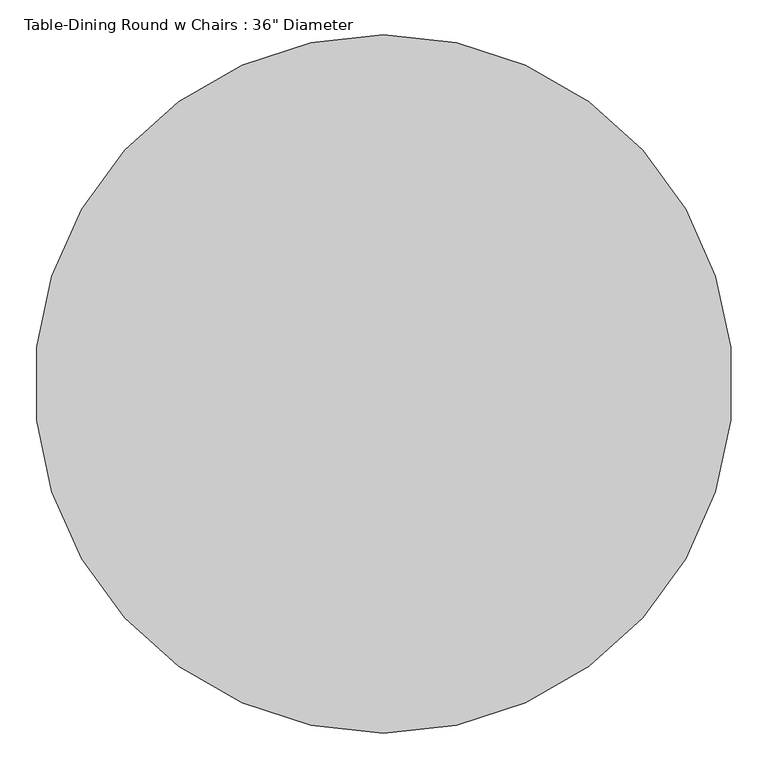
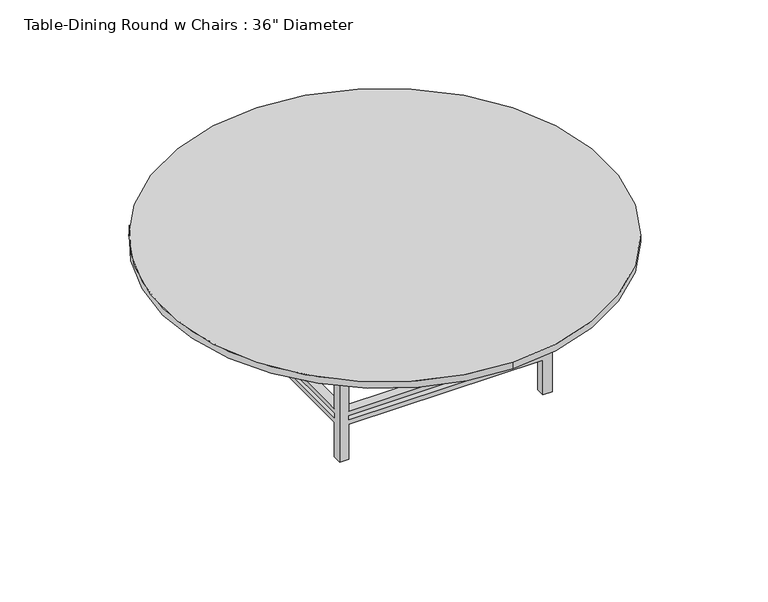
"""IFC4 building model written with IfcOpenShell, lengths in millimetres: furniture geometry."""

from ifc_helpers import new_model, si_unit, point, frame, frame_2d, origin, place, context, project, spatial, polyline, circle_curve, trimmed, segment, composite_curve, outline, extrude, faceted_brep, source, transform, mapped, element, save


def furniture_5d3b8c6f(model_context):
    return source(origin(), model_context, "Body", "SolidModel", [
        faceted_brep([(637.0819672, 348.5213115, 279.4), (637.0819672, -718.2786885, 279.4), (687.8819672, -718.2786885, 279.4), (687.8819672, 348.5213115, 279.4), (-429.7180328, -718.2786885, 279.4), (-429.7180328, -769.0786885, 279.4), (637.0819672, -769.0786885, 279.4), (-429.7180328, 348.5213115, 279.4), (-480.5180328, 348.5213115, 279.4), (-480.5180328, -718.2786885, 279.4), (637.0819672, 399.3213115, 279.4), (-429.7180328, 399.3213115, 279.4), (637.0819672, 348.5213115, 254.0), (-429.7180328, 348.5213115, 254.0), (-429.7180328, 399.3213115, 254.0), (637.0819672, 399.3213115, 254.0), (-429.7180328, -718.2786885, 254.0), (-480.5180328, -718.2786885, 254.0), (-480.5180328, 348.5213115, 254.0), (637.0819672, -718.2786885, 254.0), (637.0819672, -769.0786885, 254.0), (-429.7180328, -769.0786885, 254.0), (687.8819672, 348.5213115, 254.0), (687.8819672, -718.2786885, 254.0), (-480.5180328, 399.3213115, 647.7), (-429.7180328, 399.3213115, 647.7), (637.0819672, 399.3213115, 647.7), (687.8819672, 399.3213115, 647.7), (687.8819672, 399.3213115, 0.0), (637.0819672, 399.3213115, 0.0), (637.0819672, 399.3213115, 203.2), (-429.7180328, 399.3213115, 203.2), (-429.7180328, 399.3213115, 0.0), (-480.5180328, 399.3213115, 0.0), (-429.7180328, 399.3213115, 228.6), (637.0819672, 399.3213115, 228.6), (-480.5180328, 348.5213115, 647.7), (-480.5180328, 348.5213115, 0.0), (-480.5180328, 348.5213115, 203.2), (-480.5180328, -718.2786885, 203.2), (-480.5180328, -718.2786885, 0.0), (-480.5180328, -769.0786885, 0.0), (-480.5180328, -769.0786885, 647.7), (-480.5180328, -718.2786885, 647.7), (-480.5180328, -718.2786885, 228.6), (-480.5180328, 348.5213115, 228.6), (687.8819672, -769.0786885, 647.7), (637.0819672, -769.0786885, 647.7), (-429.7180328, -769.0786885, 647.7), (-429.7180328, -769.0786885, 0.0), (-429.7180328, -769.0786885, 203.2), (637.0819672, -769.0786885, 203.2), (637.0819672, -769.0786885, 0.0), (687.8819672, -769.0786885, 0.0), (637.0819672, -769.0786885, 228.6), (-429.7180328, -769.0786885, 228.6), (687.8819672, 348.5213115, 647.7), (687.8819672, -718.2786885, 647.7), (687.8819672, -718.2786885, 0.0), (687.8819672, -718.2786885, 203.2), (687.8819672, 348.5213115, 203.2), (687.8819672, 348.5213115, 0.0), (687.8819672, 348.5213115, 228.6), (687.8819672, -718.2786885, 228.6), (-429.7180328, 348.5213115, 647.7), (637.0819672, -718.2786885, 647.7), (637.0819672, 348.5213115, 647.7), (-429.7180328, -718.2786885, 647.7), (637.0819672, 348.5213115, 0.0), (-429.7180328, -718.2786885, 0.0), (-429.7180328, 348.5213115, 0.0), (637.0819672, -718.2786885, 0.0), (-429.7180328, 348.5213115, 228.6), (-429.7180328, 348.5213115, 203.2), (637.0819672, 348.5213115, 228.6), (637.0819672, 348.5213115, 203.2), (637.0819672, -718.2786885, 228.6), (637.0819672, -718.2786885, 203.2), (-429.7180328, -718.2786885, 228.6), (-429.7180328, -718.2786885, 203.2)], [[[0, 1, 2, 3]], [[1, 4, 5, 6]], [[4, 7, 8, 9]], [[7, 0, 10, 11]], [[12, 13, 14, 15]], [[13, 16, 17, 18]], [[16, 19, 20, 21]], [[19, 12, 22, 23]], [[24, 25, 11, 10, 26, 27, 28, 29, 30, 31, 32, 33], [14, 34, 35, 15]], [[36, 24, 33, 37, 38, 39, 40, 41, 42, 43, 9, 8], [17, 44, 45, 18]], [[46, 47, 6, 5, 48, 42, 41, 49, 50, 51, 52, 53], [20, 54, 55, 21]], [[28, 27, 56, 3, 2, 57, 46, 53, 58, 59, 60, 61], [22, 62, 63, 23]], [[1, 0, 12, 19]], [[4, 1, 19, 16]], [[7, 4, 16, 13]], [[0, 7, 13, 12]], [[25, 24, 36, 64]], [[47, 46, 57, 65]], [[26, 66, 56, 27]], [[48, 67, 43, 42]], [[29, 28, 61, 68]], [[49, 41, 40, 69]], [[32, 70, 37, 33]], [[52, 71, 58, 53]], [[13, 18, 45, 72]], [[64, 36, 8, 7]], [[37, 70, 73, 38]], [[14, 13, 72, 34]], [[25, 64, 7, 11]], [[70, 32, 31, 73]], [[12, 15, 35, 74]], [[66, 26, 10, 0]], [[29, 68, 75, 30]], [[22, 12, 74, 62]], [[56, 66, 0, 3]], [[68, 61, 60, 75]], [[19, 23, 63, 76]], [[65, 57, 2, 1]], [[58, 71, 77, 59]], [[20, 19, 76, 54]], [[47, 65, 1, 6]], [[71, 52, 51, 77]], [[16, 21, 55, 78]], [[67, 48, 5, 4]], [[49, 69, 79, 50]], [[17, 16, 78, 44]], [[43, 67, 4, 9]], [[69, 40, 39, 79]], [[74, 76, 63, 62]], [[76, 78, 55, 54]], [[78, 72, 45, 44]], [[72, 74, 35, 34]], [[75, 73, 31, 30]], [[73, 79, 39, 38]], [[79, 77, 51, 50]], [[77, 75, 60, 59]], [[76, 74, 75, 77]], [[78, 76, 77, 79]], [[72, 78, 79, 73]], [[74, 72, 73, 75]]]),
        extrude(outline(polyline([(713.2819672, 424.7213115), (713.2819672, -794.4786885), (-505.9180328, -794.4786885), (-505.9180328, 424.7213115), (713.2819672, 424.7213115)]), holes=[polyline([(687.8819672, 399.3213115), (-480.5180328, 399.3213115), (-480.5180328, -769.0786885), (687.8819672, -769.0786885), (687.8819672, 399.3213115)])]), frame((0.0, 0.0, 647.7), z_axis=(0.0, 0.0, 1.0), x_axis=(1.0, 0.0, 0.0)), (0.0, 0.0, 1.0), 76.2),
        extrude(outline(composite_curve([segment(trimmed(circle_curve(frame_2d((103.6819672, -184.8786885)), 1219.2), [point((103.6819672, -1404.0786885))], [point((103.6819672, 1034.3213115))], False, "CARTESIAN"), True, "CONTINUOUS"), segment(trimmed(circle_curve(frame_2d((103.6819672, -184.8786885)), 1219.2), [point((103.6819672, 1034.3213115))], [point((103.6819672, -1404.0786885))], False, "CARTESIAN"), True, "CONTINUOUS")], self_intersect=False)), frame((0.0, 0.0, 723.9), z_axis=(0.0, 0.0, 1.0), x_axis=(1.0, 0.0, 0.0)), (0.0, 0.0, 1.0), 38.1),
    ])


if __name__ == "__main__":
    model = new_model("IFC4")
    model_context = context("Model", 3, world=origin())
    ifc_project = project(units=[si_unit("LENGTHUNIT", "METRE", prefix="MILLI")], contexts=[model_context])
    site = spatial("IfcSite", under=ifc_project)
    building = spatial("IfcBuilding", under=site)
    placement = place(None, origin())
    furniture_shape = furniture_5d3b8c6f(model_context)
    element("IfcFurniture", 1, ObjectType="Table-Dining Round w Chairs : 36\" Diameter", at=placement, inside=building, context=model_context, shape_type="MappedRepresentation", body=[
        mapped(furniture_shape, transform((0.0, 0.0, 0.0), x_axis=(1.0, 0.0, 0.0), y_axis=(0.0, 1.0, 0.0), z_axis=(0.0, 0.0, 1.0))),
    ])
    save(model, "model.ifc")

# Revit data of these elements
# Type "Table-Dining Round w Chairs : 36\" Diameter"
#   Assembly Code = "E2020200"
#   Radius = 4' - 0"
#   Diameter = 8' - 0"
#   Height = 2' - 6"
#   Chairs = 8
#   Base Material = Pine
#   Top Material = Laminate, Linen, Matte
#   Default Elevation = 0
# Element 1 (IfcFurniture, "Table-Dining Round w Chairs : 36\" Diameter")
#   Materials on its faces: "Pine", "Laminate, Linen, Matte"
# Materials
#   "Pine": class "Wood", colour RGB 223 192 134, transparency 0, Description = "Pinus Echinata", Cost = 0
#   "Laminate, Linen, Matte": class "Plastic", colour RGB 249 239 230, transparency 0, Description = "Plastic Laminate - Linen, Matte", Cost = 0
